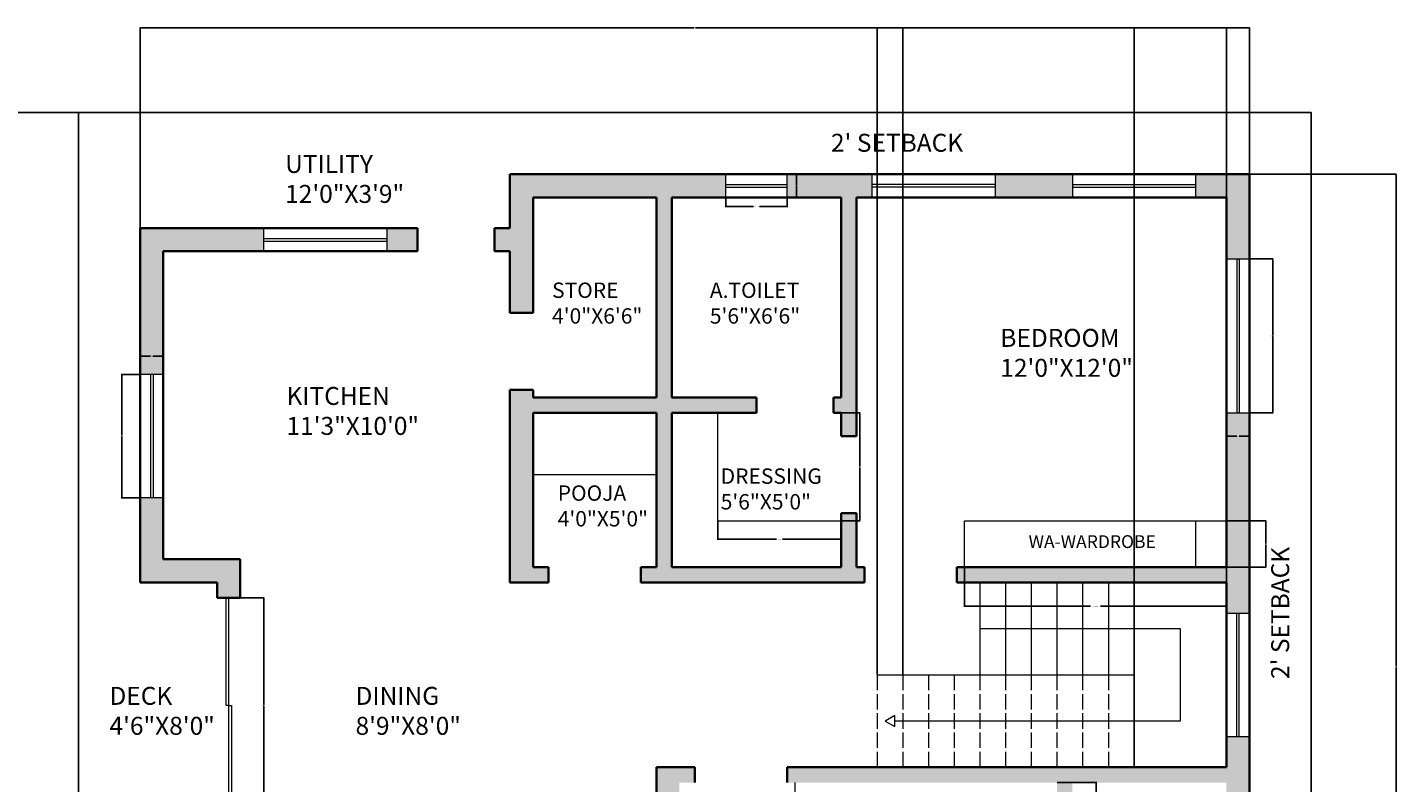
# Model space of a CAD drawing. Units: inches. Extents: x 3386 to 4477, y 1118 to 1824.
# Tile 7 of 7: x 3944 to 4477, y 1530 to 1824. Entities that reach past the tile are written whole.
import ezdxf

# ---------------------------------------------------------------- set-up
doc = ezdxf.new("R2010")
doc.units = ezdxf.units.IN
doc.linetypes.add('ACAD_ISO02W100', pattern=[15, 12, -3])
for name, color, linetype, lineweight in [('A-ANNO-DIMS', 2, 'Continuous', 18), ('A-ANNO-SYMB', 7, 'Continuous', 18), ('A-ANNO-TEXT', 7, 'Continuous', 18), ('A-AREA-IDEN', 7, 'Continuous', 18), ('A-DOOR', 4, 'Continuous', 18), ('A-FLOR-CASE', 7, 'Continuous', 18), ('A-FLOR-STRS', 7, 'Continuous', 18), ('A-FLOR-STRS-HIDN', 7, 'ACAD_ISO02W100', 13), ('A-GLAZ', 4, 'Continuous', 18), ('A-WALL', 7, 'Continuous', 35), ('C-PROP', 7, 'Continuous', 25)]:
    doc.layers.add(name, color=color, linetype=linetype, lineweight=lineweight)
doc.layers.add('A-WALL-PATT', color=18, linetype='Continuous', lineweight=13, true_color=0x000000)
doc.styles.get("Standard").update_dxf_attribs({"font": 'arial.ttf'})
doc.dimstyles.get("Standard").update_dxf_attribs({"dimtxt": 0.18, "dimasz": 0.18, "dimexe": 0.18, "dimexo": 0.0625, "dimgap": 0.09, "dimtad": 0, "dimtih": 1, "dimtoh": 1, "dimdec": 4, "dimzin": 0, "dimdsep": 46, "dimtxsty": 'Standard', "dimcen": 0.09, "dimadec": 0, "dimazin": 0, "dimtfac": 1, "dimtdec": 4, "dimtofl": 0, "dimtmove": 0, "dimatfit": 3, "dimfxl": 1, "dimtolj": 1, "dimtzin": 0, "dimarcsym": 0})

# ---------------------------------------------------------------- blocks, each defined once
blk = doc.blocks.new('WIN-24IN')
for p, q in [((0, 0), (0, 9)), ((24, 0), (24, 9)), ((0, 5), (24, 5)), ((0, 4), (24, 4))]:
    blk.add_line(p, q)
blk = doc.blocks.new('WIN-48IN')
for p, q in [((0, 48), (9, 48)), ((4, 0), (4, 48)), ((5, 0), (5, 48)), ((0, 0), (9, 0))]:
    blk.add_line(p, q)
blk = doc.blocks.new('WIN-60IN')
for p, q in [((0, 60), (9, 60)), ((4, 60), (4, 0)), ((5, 60), (5, 0)), ((0, 0), (9, 0))]:
    blk.add_line(p, q)
blk = doc.blocks.new('DOOR-SLIDING-84IN')
for p, q in [((0, 42), (0, 84)), ((1, 84), (1, 0)), ((1, 42), (0, 42)), ((1, 42), (2, 42)), ((2, 42), (2, 0))]:
    blk.add_line(p, q)
blk = doc.blocks.new('STAIR-DIRECTION')
blk.add_lwpolyline([(36.88, 38.16), (114.88, 38.16), (114.88, 2.16), (3.74, 2.16)])
blk.add_lwpolyline([(0, 2.16), (3.74, 0), (3.74, 4.32)], close=True)
blk = doc.blocks.new('WARDROBE-102IN')
for q in [(0, 18), (102, 0)]:
    blk.add_line((0, 0), q)
blk = doc.blocks.new('WARDROBE-102IN-DIVIDED')
for p, q in [((0, 18), (102, 18)), ((0, 0), (0, 18)), ((90, 18), (90, 0))]:
    blk.add_line(p, q)
blk = doc.blocks.new('DRESSING-UNIT-48X42')
for q in [(0, 42), (48, 0)]:
    blk.add_line((0, 0), q)
blk = doc.blocks.new('*D43')
at = {"layer": 'A-ANNO-DIMS', "color": 0, "lineweight": -2, "transparency": 16777216}
for p, q in [((3987.65, 1688.87), (3980.33, 1688.87)), ((3980.51, 1688.69), (3980.51, 1665.05)), ((3980.51, 1641.05), (3980.51, 1664.68)), ((3987.65, 1640.87), (3980.33, 1640.87))]:
    blk.add_line(p, q, dxfattribs=at)
at = {"layer": 'A-ANNO-DIMS', "color": 0, "transparency": 16777216}
for points in [[(3980.48, 1688.69), (3980.54, 1688.69), (3980.51, 1688.87)], [(3980.48, 1641.05), (3980.54, 1641.05), (3980.51, 1640.87)]]:
    blk.add_solid(points, dxfattribs=at)
at = {"layer": 'Defpoints', "color": 0, "transparency": 16777216}
for p in [(3987.71, 1688.87), (3980.51, 1640.87), (3987.71, 1640.87)]:
    blk.add_point(p, dxfattribs=at)
at = {"layer": 'A-ANNO-DIMS', "color": 0, "transparency": 16777216, "insert": (3980.51, 1664.87), "char_height": 0.18, "attachment_point": 5}
blk.add_mtext('\\A1;WINDOW 48 TYP.', dxfattribs=at)
blk = doc.blocks.new('*D44')
at = {"layer": 'A-ANNO-DIMS', "color": 0, "lineweight": -2, "transparency": 16777216}
for p, q in [((3987.71, 1688.93), (3987.71, 1696.25)), ((3987.89, 1696.07), (3991.75, 1696.07)), ((3996.53, 1696.07), (3992.67, 1696.07)), ((3996.71, 1688.93), (3996.71, 1696.25))]:
    blk.add_line(p, q, dxfattribs=at)
at = {"layer": 'A-ANNO-DIMS', "color": 0, "transparency": 16777216}
for points in [[(3987.89, 1696.1), (3987.89, 1696.04), (3987.71, 1696.07)], [(3996.53, 1696.1), (3996.53, 1696.04), (3996.71, 1696.07)]]:
    blk.add_solid(points, dxfattribs=at)
at = {"layer": 'Defpoints', "color": 0, "transparency": 16777216}
for p in [(3987.71, 1696.07), (3987.71, 1688.87), (3996.71, 1688.87)]:
    blk.add_point(p, dxfattribs=at)
at = {"layer": 'A-ANNO-DIMS', "color": 0, "transparency": 16777216, "insert": (3992.21, 1696.07), "char_height": 0.18, "attachment_point": 5}
blk.add_mtext('\\A1;9 TYP.', dxfattribs=at)
blk = doc.blocks.new('*D45')
at = {"layer": 'A-ANNO-DIMS', "color": 0, "lineweight": -2, "transparency": 16777216}
for p, q in [((4215.71, 1757.81), (4215.71, 1754.09)), ((4215.89, 1754.27), (4226.59, 1754.27)), ((4239.53, 1754.27), (4228.83, 1754.27)), ((4239.71, 1757.81), (4239.71, 1754.09))]:
    blk.add_line(p, q, dxfattribs=at)
at = {"layer": 'A-ANNO-DIMS', "color": 0, "transparency": 16777216}
for points in [[(4215.89, 1754.3), (4215.89, 1754.24), (4215.71, 1754.27)], [(4239.53, 1754.3), (4239.53, 1754.24), (4239.71, 1754.27)]]:
    blk.add_solid(points, dxfattribs=at)
at = {"layer": 'Defpoints', "color": 0, "transparency": 16777216}
for p in [(4215.71, 1757.87), (4239.71, 1757.87), (4239.71, 1754.27)]:
    blk.add_point(p, dxfattribs=at)
at = {"layer": 'A-ANNO-DIMS', "color": 0, "transparency": 16777216, "insert": (4227.71, 1754.27), "char_height": 0.18, "attachment_point": 5}
blk.add_mtext('\\A1;WINDOW 24 TYP.', dxfattribs=at)
blk = doc.blocks.new('*D46')
at = {"layer": 'A-ANNO-DIMS', "color": 0, "lineweight": -2, "transparency": 16777216}
for p, q in [((4239.77, 1766.87), (4243.49, 1766.87)), ((4243.31, 1766.69), (4243.31, 1762.55)), ((4243.31, 1758.05), (4243.31, 1762.19)), ((4239.77, 1757.87), (4243.49, 1757.87))]:
    blk.add_line(p, q, dxfattribs=at)
at = {"layer": 'A-ANNO-DIMS', "color": 0, "transparency": 16777216}
for points in [[(4243.28, 1766.69), (4243.34, 1766.69), (4243.31, 1766.87)], [(4243.28, 1758.05), (4243.34, 1758.05), (4243.31, 1757.87)]]:
    blk.add_solid(points, dxfattribs=at)
at = {"layer": 'Defpoints', "color": 0, "transparency": 16777216}
for p in [(4239.71, 1766.87), (4243.31, 1766.87), (4239.71, 1757.87)]:
    blk.add_point(p, dxfattribs=at)
at = {"layer": 'A-ANNO-DIMS', "color": 0, "transparency": 16777216, "insert": (4243.31, 1762.37), "char_height": 0.18, "attachment_point": 5}
blk.add_mtext('\\A1;9 TYP.', dxfattribs=at)
blk = doc.blocks.new('*D49')
at = {"layer": 'A-ANNO-DIMS', "color": 0, "lineweight": -2, "transparency": 16777216}
for p, q in [((4419.77, 1733.87), (4428.89, 1733.87)), ((4428.71, 1733.69), (4428.71, 1704.05)), ((4428.71, 1674.05), (4428.71, 1703.68)), ((4419.77, 1673.87), (4428.89, 1673.87))]:
    blk.add_line(p, q, dxfattribs=at)
at = {"layer": 'A-ANNO-DIMS', "color": 0, "transparency": 16777216}
for points in [[(4428.68, 1733.69), (4428.74, 1733.69), (4428.71, 1733.87)], [(4428.68, 1674.05), (4428.74, 1674.05), (4428.71, 1673.87)]]:
    blk.add_solid(points, dxfattribs=at)
at = {"layer": 'Defpoints', "color": 0, "transparency": 16777216}
for p in [(4419.71, 1733.87), (4428.71, 1733.87), (4419.71, 1673.87)]:
    blk.add_point(p, dxfattribs=at)
at = {"layer": 'A-ANNO-DIMS', "color": 0, "transparency": 16777216, "insert": (4428.71, 1703.87), "char_height": 0.18, "attachment_point": 5}
blk.add_mtext('\\A1;WINDOW 60 TYP.', dxfattribs=at)
blk = doc.blocks.new('*D50')
at = {"layer": 'A-ANNO-DIMS', "color": 0, "lineweight": -2, "transparency": 16777216}
for p, q in [((4410.71, 1673.81), (4410.71, 1664.69)), ((4419.71, 1673.81), (4419.71, 1664.69)), ((4410.89, 1664.87), (4414.75, 1664.87)), ((4419.53, 1664.87), (4415.67, 1664.87))]:
    blk.add_line(p, q, dxfattribs=at)
at = {"layer": 'A-ANNO-DIMS', "color": 0, "transparency": 16777216}
for points in [[(4410.89, 1664.9), (4410.89, 1664.84), (4410.71, 1664.87)], [(4419.53, 1664.9), (4419.53, 1664.84), (4419.71, 1664.87)]]:
    blk.add_solid(points, dxfattribs=at)
at = {"layer": 'Defpoints', "color": 0, "transparency": 16777216}
for p in [(4410.71, 1673.87), (4419.71, 1673.87), (4419.71, 1664.87)]:
    blk.add_point(p, dxfattribs=at)
at = {"layer": 'A-ANNO-DIMS', "color": 0, "transparency": 16777216, "insert": (4415.21, 1664.87), "char_height": 0.18, "attachment_point": 5}
blk.add_mtext('\\A1;9 TYP.', dxfattribs=at)
blk = doc.blocks.new('*D51')
at = {"layer": 'A-ANNO-DIMS', "color": 0, "lineweight": -2, "transparency": 16777216}
for p, q in [((4023.27, 1601.87), (4035.99, 1601.87)), ((4035.81, 1601.69), (4035.81, 1560.05)), ((4035.81, 1518.05), (4035.81, 1559.68)), ((4023.27, 1517.87), (4035.99, 1517.87))]:
    blk.add_line(p, q, dxfattribs=at)
at = {"layer": 'A-ANNO-DIMS', "color": 0, "transparency": 16777216}
for points in [[(4035.78, 1601.69), (4035.84, 1601.69), (4035.81, 1601.87)], [(4035.78, 1518.05), (4035.84, 1518.05), (4035.81, 1517.87)]]:
    blk.add_solid(points, dxfattribs=at)
at = {"layer": 'Defpoints', "color": 0, "transparency": 16777216}
for p in [(4023.21, 1601.87), (4023.21, 1517.87), (4035.81, 1517.87)]:
    blk.add_point(p, dxfattribs=at)
at = {"layer": 'A-ANNO-DIMS', "color": 0, "transparency": 16777216, "insert": (4035.81, 1559.87), "char_height": 0.18, "attachment_point": 5}
blk.add_mtext('\\A1;SLIDER 84 TYP.', dxfattribs=at)
blk = doc.blocks.new('*D56')
at = {"layer": 'A-ANNO-DIMS', "color": 0, "lineweight": -2, "transparency": 16777216}
for p, q in [((4344.77, 1529.87), (4360.19, 1529.87)), ((4360.01, 1529.69), (4360.01, 1521.05)), ((4360.01, 1512.05), (4360.01, 1520.69)), ((4344.77, 1511.87), (4360.19, 1511.87))]:
    blk.add_line(p, q, dxfattribs=at)
at = {"layer": 'A-ANNO-DIMS', "color": 0, "transparency": 16777216}
for points in [[(4359.98, 1529.69), (4360.04, 1529.69), (4360.01, 1529.87)], [(4359.98, 1512.05), (4360.04, 1512.05), (4360.01, 1511.87)]]:
    blk.add_solid(points, dxfattribs=at)
at = {"layer": 'Defpoints', "color": 0, "transparency": 16777216}
for p in [(4344.71, 1529.87), (4360.01, 1529.87), (4344.71, 1511.87)]:
    blk.add_point(p, dxfattribs=at)
at = {"layer": 'A-ANNO-DIMS', "color": 0, "transparency": 16777216, "insert": (4360.01, 1520.87), "char_height": 0.18, "attachment_point": 5}
blk.add_mtext('\\A1;18 TYP.', dxfattribs=at)
blk = doc.blocks.new('*D57')
at = {"layer": 'A-ANNO-DIMS', "color": 0, "lineweight": -2, "transparency": 16777216}
for p, q in [((4308.71, 1613.81), (4308.71, 1598.39)), ((4410.71, 1613.81), (4410.71, 1598.39)), ((4308.89, 1598.57), (4357.8, 1598.57)), ((4410.53, 1598.57), (4361.62, 1598.57))]:
    blk.add_line(p, q, dxfattribs=at)
at = {"layer": 'A-ANNO-DIMS', "color": 0, "transparency": 16777216}
for points in [[(4308.89, 1598.6), (4308.89, 1598.54), (4308.71, 1598.57)], [(4410.53, 1598.6), (4410.53, 1598.54), (4410.71, 1598.57)]]:
    blk.add_solid(points, dxfattribs=at)
at = {"layer": 'Defpoints', "color": 0, "transparency": 16777216}
for p in [(4308.71, 1613.87), (4410.71, 1613.87), (4410.71, 1598.57)]:
    blk.add_point(p, dxfattribs=at)
at = {"layer": 'A-ANNO-DIMS', "color": 0, "transparency": 16777216, "insert": (4359.71, 1598.57), "char_height": 0.18, "attachment_point": 5}
blk.add_mtext('\\A1;DIVIDED WARDROBE 102 TYP.', dxfattribs=at)
blk = doc.blocks.new('*D58')
at = {"layer": 'A-ANNO-DIMS', "color": 0, "lineweight": -2, "transparency": 16777216}
for p, q in [((4410.77, 1631.87), (4426.19, 1631.87)), ((4426.01, 1631.69), (4426.01, 1623.05)), ((4426.01, 1614.05), (4426.01, 1622.69)), ((4410.77, 1613.87), (4426.19, 1613.87))]:
    blk.add_line(p, q, dxfattribs=at)
at = {"layer": 'A-ANNO-DIMS', "color": 0, "transparency": 16777216}
for points in [[(4425.98, 1631.69), (4426.04, 1631.69), (4426.01, 1631.87)], [(4425.98, 1614.05), (4426.04, 1614.05), (4426.01, 1613.87)]]:
    blk.add_solid(points, dxfattribs=at)
at = {"layer": 'Defpoints', "color": 0, "transparency": 16777216}
for p in [(4410.71, 1631.87), (4426.01, 1631.87), (4410.71, 1613.87)]:
    blk.add_point(p, dxfattribs=at)
at = {"layer": 'A-ANNO-DIMS', "color": 0, "transparency": 16777216, "insert": (4426.01, 1622.87), "char_height": 0.18, "attachment_point": 5}
blk.add_mtext('\\A1;18 TYP.', dxfattribs=at)
blk = doc.blocks.new('*D59')
at = {"layer": 'A-ANNO-DIMS', "color": 0, "lineweight": -2, "transparency": 16777216}
for p, q in [((4212.71, 1631.81), (4212.71, 1624.49)), ((4260.71, 1631.81), (4260.71, 1624.49)), ((4212.89, 1624.67), (4235.54, 1624.67)), ((4260.53, 1624.67), (4237.88, 1624.67))]:
    blk.add_line(p, q, dxfattribs=at)
at = {"layer": 'A-ANNO-DIMS', "color": 0, "transparency": 16777216}
for points in [[(4212.89, 1624.7), (4212.89, 1624.64), (4212.71, 1624.67)], [(4260.53, 1624.7), (4260.53, 1624.64), (4260.71, 1624.67)]]:
    blk.add_solid(points, dxfattribs=at)
at = {"layer": 'Defpoints', "color": 0, "transparency": 16777216}
for p in [(4212.71, 1631.87), (4260.71, 1631.87), (4260.71, 1624.67)]:
    blk.add_point(p, dxfattribs=at)
at = {"layer": 'A-ANNO-DIMS', "color": 0, "transparency": 16777216, "insert": (4236.71, 1624.67), "char_height": 0.18, "attachment_point": 5}
blk.add_mtext('\\A1;DRESSER 48 TYP.', dxfattribs=at)
blk = doc.blocks.new('*D60')
at = {"layer": 'A-ANNO-DIMS', "color": 0, "lineweight": -2, "transparency": 16777216}
for p, q in [((4260.77, 1673.87), (4268.09, 1673.87)), ((4267.91, 1673.69), (4267.91, 1653.05)), ((4267.91, 1632.05), (4267.91, 1652.69)), ((4260.77, 1631.87), (4268.09, 1631.87))]:
    blk.add_line(p, q, dxfattribs=at)
at = {"layer": 'A-ANNO-DIMS', "color": 0, "transparency": 16777216}
for points in [[(4267.88, 1673.69), (4267.94, 1673.69), (4267.91, 1673.87)], [(4267.88, 1632.05), (4267.94, 1632.05), (4267.91, 1631.87)]]:
    blk.add_solid(points, dxfattribs=at)
at = {"layer": 'Defpoints', "color": 0, "transparency": 16777216}
for p in [(4260.71, 1673.87), (4267.91, 1673.87), (4260.71, 1631.87)]:
    blk.add_point(p, dxfattribs=at)
at = {"layer": 'A-ANNO-DIMS', "color": 0, "transparency": 16777216, "insert": (4267.91, 1652.87), "char_height": 0.18, "attachment_point": 5}
blk.add_mtext('\\A1;42 TYP.', dxfattribs=at)
blk = doc.blocks.new('*D106')
at = {"layer": 'A-ANNO-DIMS', "color": 0, "lineweight": -2, "transparency": 16777216}
for p, q in [((3963.65, 1790.87), (3930.48, 1790.87)), ((3930.66, 1790.69), (3930.66, 1491.05)), ((3930.66, 1191.05), (3930.66, 1490.69)), ((3963.65, 1190.87), (3930.48, 1190.87))]:
    blk.add_line(p, q, dxfattribs=at)
at = {"layer": 'A-ANNO-DIMS', "color": 0, "transparency": 16777216}
for points in [[(3930.63, 1790.69), (3930.69, 1790.69), (3930.66, 1790.87)], [(3930.63, 1191.05), (3930.69, 1191.05), (3930.66, 1190.87)]]:
    blk.add_solid(points, dxfattribs=at)
at = {"layer": 'Defpoints', "color": 0, "transparency": 16777216}
for p in [(3930.66, 1790.87), (3963.71, 1790.87), (3963.71, 1190.87)]:
    blk.add_point(p, dxfattribs=at)
at = {"layer": 'A-ANNO-DIMS', "color": 0, "transparency": 16777216, "insert": (3930.66, 1490.87), "char_height": 0.18, "attachment_point": 5}
blk.add_mtext('\\A1;600', dxfattribs=at)
blk = doc.blocks.new('*D107')
at = {"layer": 'A-ANNO-DIMS', "color": 0, "lineweight": -2, "transparency": 16777216}
for p, q in [((3987.71, 1745.93), (3987.71, 1824.1)), ((3987.89, 1823.92), (4203.42, 1823.92)), ((4419.53, 1823.92), (4204, 1823.92)), ((4419.71, 1766.93), (4419.71, 1824.1))]:
    blk.add_line(p, q, dxfattribs=at)
at = {"layer": 'A-ANNO-DIMS', "color": 0, "transparency": 16777216}
for points in [[(3987.89, 1823.95), (3987.89, 1823.89), (3987.71, 1823.92)], [(4419.53, 1823.95), (4419.53, 1823.89), (4419.71, 1823.92)]]:
    blk.add_solid(points, dxfattribs=at)
at = {"layer": 'Defpoints', "color": 0, "transparency": 16777216}
for p in [(4419.71, 1823.92), (4419.71, 1766.87), (3987.71, 1745.87)]:
    blk.add_point(p, dxfattribs=at)
at = {"layer": 'A-ANNO-DIMS', "color": 0, "transparency": 16777216, "insert": (4203.71, 1823.92), "char_height": 0.18, "attachment_point": 5}
blk.add_mtext('\\A1;432', dxfattribs=at)
blk = doc.blocks.new('*D111')
at = {"layer": 'A-ANNO-DIMS', "color": 0, "lineweight": -2, "transparency": 16777216}
for p, q in [((4419.77, 1766.87), (4476.94, 1766.87)), ((4476.76, 1766.69), (4476.76, 1575.05)), ((4476.76, 1383.05), (4476.76, 1574.69)), ((4419.77, 1382.87), (4476.94, 1382.87))]:
    blk.add_line(p, q, dxfattribs=at)
at = {"layer": 'A-ANNO-DIMS', "color": 0, "transparency": 16777216}
for points in [[(4476.73, 1766.69), (4476.79, 1766.69), (4476.76, 1766.87)], [(4476.73, 1383.05), (4476.79, 1383.05), (4476.76, 1382.87)]]:
    blk.add_solid(points, dxfattribs=at)
at = {"layer": 'Defpoints', "color": 0, "transparency": 16777216}
for p in [(4419.71, 1766.87), (4476.76, 1766.87), (4419.71, 1382.87)]:
    blk.add_point(p, dxfattribs=at)
at = {"layer": 'A-ANNO-DIMS', "color": 0, "transparency": 16777216, "insert": (4476.76, 1574.87), "char_height": 0.18, "attachment_point": 5}
blk.add_mtext('\\A1;384', dxfattribs=at)
blk = doc.blocks.new('*D112')
at = {"layer": 'A-ANNO-DIMS', "color": 0, "lineweight": -2, "transparency": 16777216}
for p, q in [((4274.71, 1571.93), (4274.71, 1824.1)), ((4274.89, 1823.92), (4279.5, 1823.92)), ((4284.53, 1823.92), (4279.92, 1823.92)), ((4284.71, 1571.93), (4284.71, 1824.1))]:
    blk.add_line(p, q, dxfattribs=at)
at = {"layer": 'A-ANNO-DIMS', "color": 0, "transparency": 16777216}
for points in [[(4274.89, 1823.95), (4274.89, 1823.89), (4274.71, 1823.92)], [(4284.53, 1823.95), (4284.53, 1823.89), (4284.71, 1823.92)]]:
    blk.add_solid(points, dxfattribs=at)
at = {"layer": 'Defpoints', "color": 0, "transparency": 16777216}
for p in [(4284.71, 1823.92), (4274.71, 1571.87), (4284.71, 1571.87)]:
    blk.add_point(p, dxfattribs=at)
at = {"layer": 'A-ANNO-DIMS', "color": 0, "transparency": 16777216, "insert": (4279.71, 1823.92), "char_height": 0.18, "attachment_point": 5}
blk.add_mtext('\\A1;10', dxfattribs=at)
blk = doc.blocks.new('*D113')
at = {"layer": 'A-ANNO-DIMS', "color": 0, "lineweight": -2, "transparency": 16777216}
for p, q in [((4374.71, 1535.93), (4374.71, 1824.1)), ((4374.89, 1823.92), (4392.49, 1823.92)), ((4410.53, 1823.92), (4392.93, 1823.92)), ((4410.71, 1535.93), (4410.71, 1824.1))]:
    blk.add_line(p, q, dxfattribs=at)
at = {"layer": 'A-ANNO-DIMS', "color": 0, "transparency": 16777216}
for points in [[(4374.89, 1823.95), (4374.89, 1823.89), (4374.71, 1823.92)], [(4410.53, 1823.95), (4410.53, 1823.89), (4410.71, 1823.92)]]:
    blk.add_solid(points, dxfattribs=at)
at = {"layer": 'Defpoints', "color": 0, "transparency": 16777216}
for p in [(4410.71, 1823.92), (4374.71, 1535.87), (4410.71, 1535.87)]:
    blk.add_point(p, dxfattribs=at)
at = {"layer": 'A-ANNO-DIMS', "color": 0, "transparency": 16777216, "insert": (4392.71, 1823.92), "char_height": 0.18, "attachment_point": 5}
blk.add_mtext('\\A1;36', dxfattribs=at)

msp = doc.modelspace()

# ---------------------------------------------------------------- hatches: boundary and pattern name
at = {"layer": 'A-WALL-PATT'}
h = msp.add_hatch(color=256, dxfattribs=at)
h.dxf.hatch_style = 1
h.paths.add_polyline_path([(4131.71, 1766.87), (4131.71, 1745.87), (4125.71, 1745.87), (4125.71, 1736.87), (4131.71, 1736.87), (4131.71, 1712.87), (4140.71, 1712.87), (4140.71, 1757.87), (4188.71, 1757.87), (4188.71, 1679.87), (4140.71, 1679.87), (4140.71, 1682.87), (4131.71, 1682.87), (4131.71, 1607.87), (4146.71, 1607.87), (4146.71, 1613.87), (4140.71, 1613.87), (4140.71, 1673.87), (4188.71, 1673.87), (4188.71, 1613.87), (4182.71, 1613.87), (4182.71, 1607.87), (4269.71, 1607.87), (4269.71, 1613.87), (4266.71, 1613.87), (4266.71, 1634.87), (4260.71, 1634.87), (4260.71, 1613.87), (4194.71, 1613.87), (4194.71, 1673.87), (4227.71, 1673.87), (4227.71, 1679.87), (4194.71, 1679.87), (4194.71, 1757.87), (4215.71, 1757.87), (4215.71, 1766.87)])
h.paths.add_polyline_path([(3987.71, 1688.87), (3996.71, 1688.87), (3996.71, 1736.87), (4035.71, 1736.87), (4035.71, 1745.87), (3987.71, 1745.87)])
h.paths.add_polyline_path([(3996.71, 1616.87), (3996.71, 1640.87), (3987.71, 1640.87), (3987.71, 1607.87), (4017.71, 1607.87), (4017.71, 1601.87), (4026.71, 1601.87), (4026.71, 1616.87)])
h.paths.add_polyline_path([(3987.71, 1511.87), (3987.71, 1478.87), (3996.71, 1478.87), (3996.71, 1502.87), (4026.71, 1502.87), (4026.71, 1517.87), (4017.71, 1517.87), (4017.71, 1511.87)])
h.paths.add_polyline_path([(3996.71, 1406.87), (3987.71, 1406.87), (3987.71, 1376.87), (3996.71, 1376.87)])
h.paths.add_polyline_path([(3996.71, 1310.87), (3996.71, 1328.87), (3987.71, 1328.87), (3987.71, 1221.87), (3996.71, 1221.87), (3996.71, 1301.87), (4002.71, 1301.87), (4002.71, 1310.87)])
h.paths.add_polyline_path([(4050.71, 1310.87), (4050.71, 1301.87), (4074.71, 1301.87), (4074.71, 1310.87)])
h.paths.add_polyline_path([(4197.71, 1301.87), (4197.71, 1382.87), (4206.71, 1382.87), (4206.71, 1391.87), (4197.71, 1391.87), (4197.71, 1529.87), (4203.71, 1529.87), (4203.71, 1535.87), (4188.71, 1535.87), (4188.71, 1310.87), (4146.71, 1310.87), (4146.71, 1301.87)])
h.paths.add_polyline_path([(4254.71, 1391.87), (4254.71, 1382.87), (4317.71, 1382.87), (4317.71, 1391.87)], flags=17)
h.paths.add_polyline_path([(4350.71, 1469.87), (4353.71, 1469.87), (4353.71, 1475.87), (4350.71, 1475.87), (4350.71, 1478.87), (4344.71, 1478.87), (4344.71, 1391.87), (4341.71, 1391.87), (4341.71, 1382.87), (4368.71, 1382.87), (4368.71, 1391.87), (4350.71, 1391.87)], flags=17)
h.paths.add_polyline_path([(4419.71, 1547.87), (4410.71, 1547.87), (4410.71, 1535.87), (4239.71, 1535.87), (4239.71, 1529.87), (4344.71, 1529.87), (4344.71, 1508.87), (4350.71, 1508.87), (4350.71, 1529.87), (4410.71, 1529.87), (4410.71, 1475.87), (4383.71, 1475.87), (4383.71, 1469.87), (4410.71, 1469.87), (4410.71, 1391.87), (4392.71, 1391.87), (4392.71, 1382.87), (4419.71, 1382.87)])
h.paths.add_polyline_path([(4419.71, 1673.87), (4410.71, 1673.87), (4410.71, 1613.87), (4305.71, 1613.87), (4305.71, 1607.87), (4410.71, 1607.87), (4410.71, 1595.87), (4419.71, 1595.87)])
h.paths.add_polyline_path([(4410.71, 1733.87), (4419.71, 1733.87), (4419.71, 1766.87), (4398.71, 1766.87), (4398.71, 1757.87), (4410.71, 1757.87)])
h.paths.add_polyline_path([(4266.71, 1757.87), (4272.71, 1757.87), (4272.71, 1766.87), (4239.71, 1766.87), (4239.71, 1757.87), (4260.71, 1757.87), (4260.71, 1679.87), (4257.71, 1679.87), (4257.71, 1673.87), (4260.71, 1673.87), (4260.71, 1664.87), (4266.71, 1664.87)])
h.paths.add_polyline_path([(4350.71, 1757.87), (4350.71, 1766.87), (4320.71, 1766.87), (4320.71, 1757.87)])
h.paths.add_polyline_path([(4083.71, 1745.87), (4083.71, 1736.87), (4095.71, 1736.87), (4095.71, 1745.87)])

# ---------------------------------------------------------------- linework, layer by layer
at = {"layer": 'A-FLOR-CASE'}
msp.add_line((4140.71, 1649.87), (4188.71, 1649.87), dxfattribs=at)
at = {"layer": 'A-FLOR-STRS'}
for p, q in [((4314.71, 1607.87), (4314.71, 1571.87)), ((4324.71, 1607.87), (4324.71, 1571.87)), ((4334.71, 1607.87), (4334.71, 1571.87)), ((4344.71, 1607.87), (4344.71, 1571.87)), ((4354.71, 1607.87), (4354.71, 1571.87)), ((4364.71, 1607.87), (4364.71, 1571.87)), ((4374.71, 1607.87), (4374.71, 1571.87)), ((4274.71, 1571.87), (4374.71, 1571.87))]:
    msp.add_line(p, q, dxfattribs=at)
at = {"layer": 'A-FLOR-STRS-HIDN', "ltscale": 0.5}
for p, q in [((4274.71, 1571.87), (4274.71, 1535.87)), ((4284.71, 1571.87), (4284.71, 1535.87)), ((4294.71, 1571.87), (4294.71, 1535.87)), ((4304.71, 1571.87), (4304.71, 1535.87)), ((4314.71, 1571.87), (4314.71, 1535.87)), ((4324.71, 1571.87), (4324.71, 1535.87)), ((4334.71, 1571.87), (4334.71, 1535.87)), ((4344.71, 1571.87), (4344.71, 1535.87)), ((4354.71, 1571.87), (4354.71, 1535.87)), ((4364.71, 1571.87), (4364.71, 1535.87)), ((4374.71, 1571.87), (4374.71, 1535.87))]:
    msp.add_line(p, q, dxfattribs=at)
at = {"layer": 'A-WALL'}
for p, q in [((4131.71, 1766.87), (4419.71, 1766.87)), ((4131.71, 1745.87), (4131.71, 1766.87)), ((4419.71, 1766.87), (4419.71, 1382.87)), ((4140.71, 1757.87), (4188.71, 1757.87)), ((4140.71, 1712.87), (4140.71, 1757.87)), ((4188.71, 1679.87), (4188.71, 1757.87)), ((4194.71, 1757.87), (4260.71, 1757.87)), ((4194.71, 1679.87), (4194.71, 1757.87)), ((4260.71, 1757.87), (4260.71, 1679.87)), ((4266.71, 1757.87), (4410.71, 1757.87)), ((4266.71, 1757.87), (4266.71, 1664.87)), ((4410.71, 1757.87), (4410.71, 1613.87)), ((3987.71, 1607.87), (3987.71, 1745.87)), ((3987.71, 1745.87), (4095.71, 1745.87)), ((4095.71, 1736.87), (4095.71, 1745.87)), ((4125.71, 1745.87), (4131.71, 1745.87)), ((4125.71, 1736.87), (4125.71, 1745.87)), ((3996.71, 1736.87), (4095.71, 1736.87)), ((3996.71, 1616.87), (3996.71, 1736.87)), ((4125.71, 1736.87), (4131.71, 1736.87)), ((4131.71, 1712.87), (4131.71, 1736.87)), ((4131.71, 1712.87), (4140.71, 1712.87)), ((4131.71, 1682.87), (4140.71, 1682.87)), ((4131.71, 1607.87), (4131.71, 1682.87)), ((4140.71, 1679.87), (4140.71, 1682.87)), ((4140.71, 1679.87), (4188.71, 1679.87)), ((4194.71, 1679.87), (4227.71, 1679.87)), ((4227.71, 1679.87), (4227.71, 1673.87)), ((4257.71, 1679.87), (4260.71, 1679.87)), ((4257.71, 1679.87), (4257.71, 1673.87)), ((4140.71, 1673.87), (4188.71, 1673.87)), ((4140.71, 1613.87), (4140.71, 1673.87)), ((4188.71, 1613.87), (4188.71, 1673.87)), ((4194.71, 1673.87), (4227.71, 1673.87)), ((4194.71, 1613.87), (4194.71, 1673.87)), ((4257.71, 1673.87), (4260.71, 1673.87)), ((4260.71, 1673.87), (4260.71, 1664.87)), ((4260.71, 1664.87), (4266.71, 1664.87)), ((4260.71, 1634.87), (4266.71, 1634.87)), ((4260.71, 1634.87), (4260.71, 1613.87)), ((4266.71, 1634.87), (4266.71, 1613.87)), ((3996.71, 1616.87), (4026.71, 1616.87)), ((4026.71, 1601.87), (4026.71, 1616.87)), ((4140.71, 1613.87), (4146.71, 1613.87)), ((4146.71, 1607.87), (4146.71, 1613.87)), ((4182.71, 1613.87), (4188.71, 1613.87)), ((4182.71, 1607.87), (4182.71, 1613.87)), ((4194.71, 1613.87), (4260.71, 1613.87)), ((4266.71, 1613.87), (4269.71, 1613.87)), ((4269.71, 1613.87), (4269.71, 1607.87)), ((4305.71, 1613.87), (4410.71, 1613.87)), ((4305.71, 1613.87), (4305.71, 1607.87)), ((3987.71, 1607.87), (4017.71, 1607.87)), ((4017.71, 1601.87), (4017.71, 1607.87)), ((4131.71, 1607.87), (4146.71, 1607.87)), ((4182.71, 1607.87), (4269.71, 1607.87)), ((4305.71, 1607.87), (4410.71, 1607.87)), ((4410.71, 1607.87), (4410.71, 1535.87)), ((4017.71, 1601.87), (4026.71, 1601.87)), ((4188.71, 1310.87), (4188.71, 1535.87)), ((4188.71, 1535.87), (4203.71, 1535.87)), ((4203.71, 1529.87), (4203.71, 1535.87)), ((4239.71, 1529.87), (4239.71, 1535.87)), ((4239.71, 1535.87), (4410.71, 1535.87))]:
    msp.add_line(p, q, dxfattribs=at)
at = {"layer": 'C-PROP'}
msp.add_lwpolyline([(3963.71, 1790.87), (4443.71, 1790.87), (4443.71, 1190.87), (3963.71, 1190.87)], close=True, dxfattribs=at)

# ---------------------------------------------------------------- block references
at = {"layer": 'A-ANNO-SYMB'}
msp.add_blockref('STAIR-DIRECTION', (4277.83, 1551.71), dxfattribs=at)
at = {"layer": 'A-DOOR', "rotation": 180}
msp.add_blockref('DOOR-SLIDING-84IN', (4023.21, 1601.87), dxfattribs=at)
at = {"layer": 'A-FLOR-CASE'}
for name, p in [('DRESSING-UNIT-48X42', (4212.71, 1631.87)), ('WARDROBE-102IN-DIVIDED', (4308.71, 1613.87)), ('WARDROBE-102IN', (4242.71, 1511.87))]:
    msp.add_blockref(name, p, dxfattribs=at)
at = {"layer": 'A-GLAZ'}
for name, p in [('WIN-24IN', (4215.71, 1757.87)), ('WIN-60IN', (4410.71, 1673.87)), ('WIN-48IN', (4410.71, 1547.87))]:
    msp.add_blockref(name, p, dxfattribs=at)
for p, rotation in [((4320.71, 1757.87), 89.99999999999763), ((4350.71, 1766.87), 270.0000000000005), ((4035.71, 1745.87), 269.9999999999987), ((3996.71, 1688.87), 180)]:
    msp.add_blockref('WIN-48IN', p, dxfattribs=dict(at, rotation=rotation))

# ---------------------------------------------------------------- texts
at = {"layer": 'A-ANNO-TEXT', "attachment_point": 1}
for s, insert, char_height in [("{\\fTimes New Roman|b0|i0|c0|p18;2' SETBACK}", (4256.7, 1782.64), 7), ('{\\fTimes New Roman|b0|i0|c0|p18;WA-WARDROBE}', (4333.66, 1626.26), 5)]:
    msp.add_mtext_dynamic_manual_height_columns(s, width=79.5604, gutter_width=12.5, heights=[0], dxfattribs=dict(at, insert=insert, char_height=char_height))
at = {"layer": 'A-ANNO-TEXT', "insert": (4428.13, 1570.24), "char_height": 7, "attachment_point": 1, "rotation": 90}
msp.add_mtext_dynamic_manual_height_columns("{\\fTimes New Roman|b0|i0|c0|p18;2' SETBACK}", width=79.5604, gutter_width=12.5, heights=[0], dxfattribs=at)
at = {"layer": 'A-AREA-IDEN', "attachment_point": 1}
for s, width, heights, insert, char_height in [('{\\fTimes New Roman|b0|i0|c0|p18;UTILITY\\P12\'0"X3\'9"}', 113.4175, [0], (4044.16, 1774.39), 7), ('{\\fTimes New Roman|b0|i0|c0|p18;STORE\\P4\'0"X6\'6"}', 79.5604, [0], (4148.1, 1724.69), 6), ('{\\fTimes New Roman|b0|i0|c0|p18;A.TOILET\\P5\'6"X6\'6"}', 79.5604, [0], (4209.54, 1724.69), 6), ('{\\fTimes New Roman|b0|i0|c0|p18;BEDROOM\\P12\'0"X12\'0"}', 79.5604, [0], (4322.64, 1706.63), 7), ('{\\fTimes New Roman|b0|i0|c0|p18;KITCHEN\\P11\'3"X10\'0"}', 79.5604, [18.79], (4044.67, 1684.01), 7), ('{\\fTimes New Roman|b0|i0|c0|p18;DRESSING\\P5\'6"X5\'0"}', 52.5784, [0], (4213.76, 1652.28), 6), ('{\\fTimes New Roman|b0|i0|c0|p18;POOJA\\P4\'0"X5\'0"}', 79.5604, [0], (4150.3, 1645.67), 6), ('{\\fTimes New Roman|b0|i0|c0|p18;DECK\\P4\'6"X8\'0"}', 79.5604, [0], (3975.75, 1567.17), 7), ('{\\fTimes New Roman|b0|i0|c0|p18;DINING\\P8\'9"X8\'0"}', 79.5604, [0], (4071.57, 1567.17), 7)]:
    msp.add_mtext_dynamic_manual_height_columns(s, width=width, gutter_width=12.5, heights=heights, dxfattribs=dict(at, insert=insert, char_height=char_height))

# ---------------------------------------------------------------- dimensions: what is measured, and where the dimension line sits
at = {"layer": 'A-ANNO-DIMS'}
for base, p1, p2, picture, middle in [((4419.71, 1823.92), (3987.71, 1745.87), (4419.71, 1766.87), '*D107', (4203.71, 1823.92)), ((4284.71, 1823.92), (4274.71, 1571.87), (4284.71, 1571.87), '*D112', (4279.71, 1823.92)), ((4410.71, 1823.92), (4374.71, 1535.87), (4410.71, 1535.87), '*D113', (4392.71, 1823.92))]:
    dim = msp.add_linear_dim(base=base, p1=p1, p2=p2, dimstyle='Standard', override={"dimdec": 0, "dimlfac": 1, "dimrnd": 0, "dimzin": 0, "dimdsep": 46, "dimlunit": 2}, dxfattribs=at)
    dim.commit()
    dim.dimension.update_dxf_attribs({"geometry": picture, "text_midpoint": middle})
for base, p1, p2, picture, middle in [((3930.66, 1790.87), (3963.71, 1190.87), (3963.71, 1790.87), '*D106', (3930.66, 1490.87)), ((4476.76, 1766.87), (4419.71, 1382.87), (4419.71, 1766.87), '*D111', (4476.76, 1574.87))]:
    dim = msp.add_linear_dim(base=base, p1=p1, p2=p2, angle=90, dimstyle='Standard', override={"dimdec": 0, "dimlfac": 1, "dimrnd": 0, "dimzin": 0, "dimdsep": 46, "dimlunit": 2}, dxfattribs=at)
    dim.commit()
    dim.dimension.update_dxf_attribs({"geometry": picture, "text_midpoint": middle})
for base, p1, p2, angle, text, picture, middle in [((4243.31, 1766.87), (4239.71, 1757.87), (4239.71, 1766.87), 90, '<> TYP.', '*D46', (4243.31, 1762.37)), ((4428.71, 1733.87), (4419.71, 1673.87), (4419.71, 1733.87), 90, 'WINDOW <> TYP.', '*D49', (4428.71, 1703.87)), ((3987.71, 1696.07), (3996.71, 1688.87), (3987.71, 1688.87), 180, '<> TYP.', '*D44', (3992.21, 1696.07)), ((3980.51, 1640.87), (3987.71, 1688.87), (3987.71, 1640.87), 270, 'WINDOW <> TYP.', '*D43', (3980.51, 1664.87)), ((4267.91, 1673.87), (4260.71, 1631.87), (4260.71, 1673.87), 90, '<> TYP.', '*D60', (4267.91, 1652.87)), ((4426.01, 1631.87), (4410.71, 1613.87), (4410.71, 1631.87), 90, '<> TYP.', '*D58', (4426.01, 1622.87)), ((4035.81, 1517.87), (4023.21, 1601.87), (4023.21, 1517.87), 270, 'SLIDER <> TYP.', '*D51', (4035.81, 1559.87)), ((4360.01, 1529.87), (4344.71, 1511.87), (4344.71, 1529.87), 90, '<> TYP.', '*D56', (4360.01, 1520.87))]:
    dim = msp.add_linear_dim(base=base, p1=p1, p2=p2, angle=angle, text=text, dimstyle='Standard', override={"dimdec": 0, "dimlfac": 1, "dimrnd": 0, "dimzin": 0, "dimdsep": 46, "dimlunit": 2}, dxfattribs=at)
    dim.commit()
    dim.dimension.update_dxf_attribs({"geometry": picture, "text_midpoint": middle})
for base, p1, p2, text, picture, middle in [((4239.71, 1754.27), (4215.71, 1757.87), (4239.71, 1757.87), 'WINDOW <> TYP.', '*D45', (4227.71, 1754.27)), ((4419.71, 1664.87), (4410.71, 1673.87), (4419.71, 1673.87), '<> TYP.', '*D50', (4415.21, 1664.87)), ((4260.71, 1624.67), (4212.71, 1631.87), (4260.71, 1631.87), 'DRESSER <> TYP.', '*D59', (4236.71, 1624.67)), ((4410.71, 1598.57), (4308.71, 1613.87), (4410.71, 1613.87), 'DIVIDED WARDROBE <> TYP.', '*D57', (4359.71, 1598.57))]:
    dim = msp.add_linear_dim(base=base, p1=p1, p2=p2, text=text, dimstyle='Standard', override={"dimdec": 0, "dimlfac": 1, "dimrnd": 0, "dimzin": 0, "dimdsep": 46, "dimlunit": 2}, dxfattribs=at)
    dim.commit()
    dim.dimension.update_dxf_attribs({"geometry": picture, "text_midpoint": middle})

doc.saveas('drawing.dxf')
